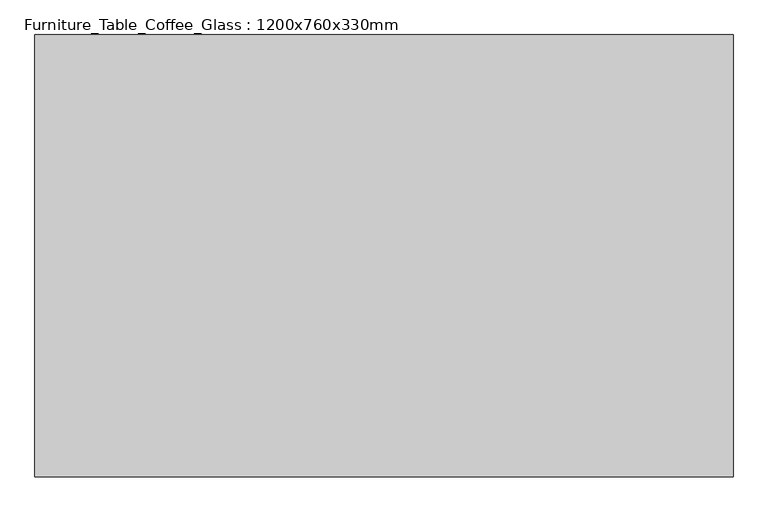
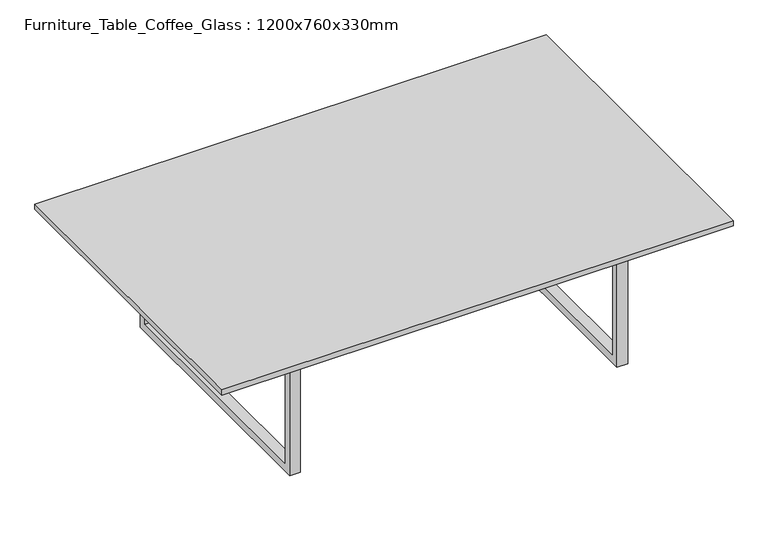
"""IFC4 building model written with IfcOpenShell, lengths in millimetres: furniture geometry, Furniture_Table_Coffee_Glass : 1200x760x330mm."""

from ifc_helpers import new_model, si_unit, frame, origin, place, context, project, spatial, polyline, outline, extrude, source, transform, mapped, element, save


def furniture_table_coffee_glass_1200x760x330mm_bccf866f(model_context):
    return source(origin(), model_context, "Body", "SweptSolid", [
        extrude(outline(polyline([(1203.7336303, 748.6108318), (1203.7336303, -11.3891682), (3.7336303, -11.3891682), (3.7336303, 748.6108318), (1203.7336303, 748.6108318)])), frame((0.0, 0.0, 317.3), z_axis=(0.0, 0.0, 1.0), x_axis=(1.0, 0.0, 0.0)), (0.0, 0.0, 1.0), 12.7),
        extrude(outline(polyline([(64.8108318, 317.3), (672.4108318, 317.3), (672.4108318, 0.0), (64.8108318, 0.0), (64.8108318, 317.3)]), holes=[polyline([(83.8608318, 298.25), (83.8608318, 19.05), (653.3608318, 19.05), (653.3608318, 298.25), (83.8608318, 298.25)])]), frame((206.9336303, 0.0, 0.0), z_axis=(1.0, 0.0, 0.0), x_axis=(0.0, 1.0, 0.0)), (0.0, 0.0, 1.0), 25.4),
        extrude(outline(polyline([(64.8108318, 317.3), (672.4108318, 317.3), (672.4108318, 0.0), (64.8108318, 0.0), (64.8108318, 317.3)]), holes=[polyline([(83.8608318, 298.25), (83.8608318, 19.05), (653.3608318, 19.05), (653.3608318, 298.25), (83.8608318, 298.25)])]), frame((975.1336303, 0.0, 0.0), z_axis=(1.0, 0.0, 0.0), x_axis=(0.0, 1.0, 0.0)), (0.0, 0.0, 1.0), 25.4),
        extrude(outline(polyline([(975.1336303, 378.1358318), (975.1336303, 359.0858318), (232.3336303, 359.0858318), (232.3336303, 378.1358318), (975.1336303, 378.1358318)])), frame((0.0, 0.0, 298.25), z_axis=(0.0, 0.0, 1.0), x_axis=(1.0, 0.0, 0.0)), (0.0, 0.0, 1.0), 19.05),
    ])


if __name__ == "__main__":
    model = new_model("IFC4")
    model_context = context("Model", 3, world=origin())
    ifc_project = project(units=[si_unit("LENGTHUNIT", "METRE", prefix="MILLI")], contexts=[model_context])
    site = spatial("IfcSite", under=ifc_project)
    building = spatial("IfcBuilding", under=site)
    placement = place(None, origin())
    furniture_table_coffee_glass_1200x760x330mm_shape = furniture_table_coffee_glass_1200x760x330mm_bccf866f(model_context)
    element("IfcFurniture", 1, ObjectType="Furniture_Table_Coffee_Glass : 1200x760x330mm", at=placement, inside=building, context=model_context, shape_type="MappedRepresentation", body=[
        mapped(furniture_table_coffee_glass_1200x760x330mm_shape, transform((0.0, 0.0, 0.0), x_axis=(1.0, 0.0, 0.0), y_axis=(0.0, 1.0, 0.0), z_axis=(0.0, 0.0, 1.0))),
    ])
    save(model, "model.ifc")

# Revit data of these elements
# Type "Furniture_Table_Coffee_Glass : 1200x760x330mm"
#   Keynote = "N"
#   Height = 1.082677 ft
#   Length = 3.937008 ft
#   Width = 2.493438 ft
#   Material Base = Metal - Chrome
#   Material Top = Glass - Clear, Grey
#   Default Elevation = 0
#   Assembly Code = ""
# Element 1 (IfcFurniture, "Furniture_Table_Coffee_Glass : 1200x760x330mm")
#   Materials on its faces: "Metal - Chrome", "Glass - Clear, Grey"
# Materials
#   "Metal - Chrome": class "Metal", colour RGB 247 247 247, transparency 0
#   "Glass - Clear, Grey": class "Glass", colour RGB 252 255 255, transparency 0.64
